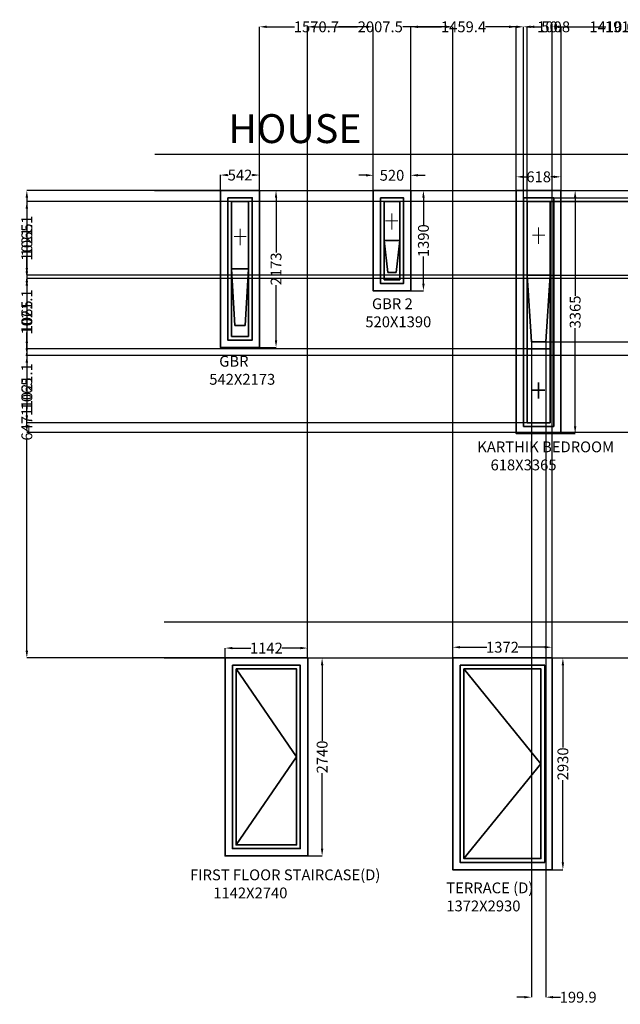
# Model space of a CAD drawing. Units: millimetres. Extents: x 16338 to 57165, y -4429 to 26237.
# Tile 1 of 6: x 16338 to 24645, y -4429 to 9199. Entities that reach past the tile are written whole.
import ezdxf

# ---------------------------------------------------------------- set-up
doc = ezdxf.new("R2010")
doc.units = ezdxf.units.MM
doc.header["$MEASUREMENT"] = 0
for name, color, linetype, lineweight in [('A-ANNO-DIMS', 5, 'Continuous', 18), ('A-ANNO-SYMB', 4, 'Continuous', 18), ('A-ANNO-TEXT', 3, 'Continuous', 18), ('A-ELEV', 8, 'Continuous', 25), ('A-GLAZ', 7, 'Continuous', 35)]:
    doc.layers.add(name, color=color, linetype=linetype, lineweight=lineweight)
doc.styles.get("Standard").update_dxf_attribs({"font": 'arial.ttf'})
doc.dimstyles.get("Standard").update_dxf_attribs({"dimtxt": 150, "dimasz": 100, "dimexe": 0.18, "dimexo": 0.0625, "dimgap": 0.09, "dimtad": 0, "dimdec": 0, "dimzin": 0, "dimdsep": 46, "dimtxsty": 'Standard', "dimcen": 0.09, "dimadec": 0, "dimazin": 0, "dimtfac": 1, "dimtdec": 0, "dimtofl": 0, "dimtmove": 0, "dimatfit": 3, "dimfxl": 1, "dimtolj": 1, "dimtzin": 0, "dimarcsym": 0})

# ---------------------------------------------------------------- blocks, each defined once
blk = doc.blocks.new('*D48')
at = {"layer": 'A-ANNO-DIMS', "color": 0, "lineweight": -2, "transparency": 16777216}
for p, q in [((19114, 6835), (19114, 7049)), ((19214, 7048), (19220, 7048)), ((19556, 7048), (19551, 7048)), ((19656, 6835), (19656, 7049))]:
    blk.add_line(p, q, dxfattribs=at)
at = {"layer": 'A-ANNO-DIMS', "color": 0, "transparency": 16777216}
for points in [[(19214, 7065), (19214, 7032), (19114, 7048)], [(19556, 7065), (19556, 7032), (19656, 7048)]]:
    blk.add_solid(points, dxfattribs=at)
at = {"layer": 'Defpoints', "color": 0, "transparency": 16777216}
for p in [(19656, 7048), (19114, 6835), (19656, 6835)]:
    blk.add_point(p, dxfattribs=at)
at = {"layer": 'A-ANNO-DIMS', "color": 0, "transparency": 16777216, "insert": (19385, 7048), "char_height": 150, "attachment_point": 5}
blk.add_mtext('\\A1;542', dxfattribs=at)
blk = doc.blocks.new('*D49')
at = {"layer": 'A-ANNO-DIMS', "color": 0, "lineweight": -2, "transparency": 16777216}
for p, q in [((19657, 6835), (19884, 6835)), ((19884, 6735), (19884, 5974)), ((19884, 4762), (19884, 5523)), ((19657, 4662), (19884, 4662))]:
    blk.add_line(p, q, dxfattribs=at)
at = {"layer": 'A-ANNO-DIMS', "color": 0, "transparency": 16777216}
for points in [[(19867, 6735), (19900, 6735), (19884, 6835)], [(19867, 4762), (19900, 4762), (19884, 4662)]]:
    blk.add_solid(points, dxfattribs=at)
at = {"layer": 'Defpoints', "color": 0, "transparency": 16777216}
for p in [(19656, 6835), (19656, 4662), (19884, 4662)]:
    blk.add_point(p, dxfattribs=at)
at = {"layer": 'A-ANNO-DIMS', "color": 0, "transparency": 16777216, "insert": (19884, 5749), "char_height": 150, "attachment_point": 5, "rotation": 90}
blk.add_mtext('\\A1;2173', dxfattribs=at)
blk = doc.blocks.new('*D50')
at = {"layer": 'A-ANNO-DIMS', "color": 0, "lineweight": -2, "transparency": 16777216}
for p, q in [((21127, 7045), (21027, 7045)), ((21227, 6835), (21227, 7045)), ((21747, 6835), (21747, 7045)), ((21847, 7045), (21947, 7045))]:
    blk.add_line(p, q, dxfattribs=at)
at = {"layer": 'A-ANNO-DIMS', "color": 0, "transparency": 16777216}
for points in [[(21127, 7062), (21127, 7028), (21227, 7045)], [(21847, 7062), (21847, 7028), (21747, 7045)]]:
    blk.add_solid(points, dxfattribs=at)
at = {"layer": 'Defpoints', "color": 0, "transparency": 16777216}
for p in [(21747, 7045), (21227, 6835), (21747, 6835)]:
    blk.add_point(p, dxfattribs=at)
at = {"layer": 'A-ANNO-DIMS', "color": 0, "transparency": 16777216, "insert": (21487, 7045), "char_height": 150, "attachment_point": 5}
blk.add_mtext('\\A1;520', dxfattribs=at)
blk = doc.blocks.new('*D51')
at = {"layer": 'A-ANNO-DIMS', "color": 0, "lineweight": -2, "transparency": 16777216}
for p, q in [((21747, 6835), (21923, 6835)), ((21922, 6735), (21922, 6357)), ((21922, 5545), (21922, 5923)), ((21747, 5445), (21923, 5445))]:
    blk.add_line(p, q, dxfattribs=at)
at = {"layer": 'A-ANNO-DIMS', "color": 0, "transparency": 16777216}
for points in [[(21906, 6735), (21939, 6735), (21922, 6835)], [(21906, 5545), (21939, 5545), (21922, 5445)]]:
    blk.add_solid(points, dxfattribs=at)
at = {"layer": 'Defpoints', "color": 0, "transparency": 16777216}
for p in [(21747, 6835), (21747, 5445), (21922, 5445)]:
    blk.add_point(p, dxfattribs=at)
at = {"layer": 'A-ANNO-DIMS', "color": 0, "transparency": 16777216, "insert": (21922, 6140), "char_height": 150, "attachment_point": 5, "rotation": 90}
blk.add_mtext('\\A1;1390', dxfattribs=at)
blk = doc.blocks.new('*D52')
at = {"layer": 'A-ANNO-DIMS', "color": 0, "lineweight": -2, "transparency": 16777216}
for p, q in [((23207, 6835), (23207, 7024)), ((23307, 7024), (23349, 7024)), ((23725, 7024), (23682, 7024)), ((23825, 6835), (23825, 7024))]:
    blk.add_line(p, q, dxfattribs=at)
at = {"layer": 'A-ANNO-DIMS', "color": 0, "transparency": 16777216}
for points in [[(23307, 7040), (23307, 7007), (23207, 7024)], [(23725, 7040), (23725, 7007), (23825, 7024)]]:
    blk.add_solid(points, dxfattribs=at)
at = {"layer": 'Defpoints', "color": 0, "transparency": 16777216}
for p in [(23825, 7024), (23207, 6835), (23825, 6835)]:
    blk.add_point(p, dxfattribs=at)
at = {"layer": 'A-ANNO-DIMS', "color": 0, "transparency": 16777216, "insert": (23516, 7024), "char_height": 150, "attachment_point": 5}
blk.add_mtext('\\A1;618', dxfattribs=at)
blk = doc.blocks.new('*D53')
at = {"layer": 'A-ANNO-DIMS', "color": 0, "lineweight": -2, "transparency": 16777216}
for p, q in [((23825, 6835), (24021, 6835)), ((24021, 6735), (24021, 5377)), ((24021, 3570), (24021, 4928)), ((23825, 3470), (24021, 3470))]:
    blk.add_line(p, q, dxfattribs=at)
at = {"layer": 'A-ANNO-DIMS', "color": 0, "transparency": 16777216}
for points in [[(24004, 6735), (24037, 6735), (24021, 6835)], [(24004, 3570), (24037, 3570), (24021, 3470)]]:
    blk.add_solid(points, dxfattribs=at)
at = {"layer": 'Defpoints', "color": 0, "transparency": 16777216}
for p in [(23825, 6835), (23825, 3470), (24021, 3470)]:
    blk.add_point(p, dxfattribs=at)
at = {"layer": 'A-ANNO-DIMS', "color": 0, "transparency": 16777216, "insert": (24021, 5153), "char_height": 150, "attachment_point": 5, "rotation": 90}
blk.add_mtext('\\A1;3365', dxfattribs=at)
blk = doc.blocks.new('*D71')
at = {"layer": 'A-ANNO-DIMS', "color": 0, "lineweight": -2, "transparency": 16777216}
for p, q in [((19179, 364), (19179, 501)), ((19279, 501), (19534, 501)), ((20221, 501), (19966, 501)), ((20321, 364), (20321, 501))]:
    blk.add_line(p, q, dxfattribs=at)
at = {"layer": 'A-ANNO-DIMS', "color": 0, "transparency": 16777216}
for points in [[(19279, 518), (19279, 485), (19179, 501)], [(20221, 518), (20221, 485), (20321, 501)]]:
    blk.add_solid(points, dxfattribs=at)
at = {"layer": 'Defpoints', "color": 0, "transparency": 16777216}
for p in [(20321, 501), (19179, 364), (20321, 364)]:
    blk.add_point(p, dxfattribs=at)
at = {"layer": 'A-ANNO-DIMS', "color": 0, "transparency": 16777216, "insert": (19750, 501), "char_height": 150, "attachment_point": 5}
blk.add_mtext('\\A1;1142', dxfattribs=at)
blk = doc.blocks.new('*D72')
at = {"layer": 'A-ANNO-DIMS', "color": 0, "lineweight": -2, "transparency": 16777216}
for p, q in [((20321, 364), (20521, 364)), ((20521, 264), (20521, -781)), ((20521, -2276), (20521, -1231)), ((20321, -2376), (20521, -2376))]:
    blk.add_line(p, q, dxfattribs=at)
at = {"layer": 'A-ANNO-DIMS', "color": 0, "transparency": 16777216}
for points in [[(20504, 264), (20538, 264), (20521, 364)], [(20504, -2276), (20538, -2276), (20521, -2376)]]:
    blk.add_solid(points, dxfattribs=at)
at = {"layer": 'Defpoints', "color": 0, "transparency": 16777216}
for p in [(20321, 364), (20321, -2376), (20521, -2376)]:
    blk.add_point(p, dxfattribs=at)
at = {"layer": 'A-ANNO-DIMS', "color": 0, "transparency": 16777216, "insert": (20521, -1006), "char_height": 150, "attachment_point": 5, "rotation": 90}
blk.add_mtext('\\A1;2740', dxfattribs=at)
blk = doc.blocks.new('*D73')
at = {"layer": 'A-ANNO-DIMS', "color": 0, "lineweight": -2, "transparency": 16777216}
for p, q in [((22329, 364), (22329, 513)), ((22429, 513), (22798, 513)), ((23601, 513), (23231, 513)), ((23701, 364), (23701, 513))]:
    blk.add_line(p, q, dxfattribs=at)
at = {"layer": 'A-ANNO-DIMS', "color": 0, "transparency": 16777216}
for points in [[(22429, 529), (22429, 496), (22329, 513)], [(23601, 529), (23601, 496), (23701, 513)]]:
    blk.add_solid(points, dxfattribs=at)
at = {"layer": 'Defpoints', "color": 0, "transparency": 16777216}
for p in [(23701, 513), (22329, 364), (23701, 364)]:
    blk.add_point(p, dxfattribs=at)
at = {"layer": 'A-ANNO-DIMS', "color": 0, "transparency": 16777216, "insert": (23015, 513), "char_height": 150, "attachment_point": 5}
blk.add_mtext('\\A1;1372', dxfattribs=at)
blk = doc.blocks.new('*D74')
at = {"layer": 'A-ANNO-DIMS', "color": 0, "lineweight": -2, "transparency": 16777216}
for p, q in [((23701, 364), (23851, 364)), ((23851, 264), (23851, -876)), ((23851, -2466), (23851, -1326)), ((23701, -2566), (23851, -2566))]:
    blk.add_line(p, q, dxfattribs=at)
at = {"layer": 'A-ANNO-DIMS', "color": 0, "transparency": 16777216}
for points in [[(23834, 264), (23867, 264), (23851, 364)], [(23834, -2466), (23867, -2466), (23851, -2566)]]:
    blk.add_solid(points, dxfattribs=at)
at = {"layer": 'Defpoints', "color": 0, "transparency": 16777216}
for p in [(23701, 364), (23701, -2566), (23851, -2566)]:
    blk.add_point(p, dxfattribs=at)
at = {"layer": 'A-ANNO-DIMS', "color": 0, "transparency": 16777216, "insert": (23851, -1101), "char_height": 150, "attachment_point": 5, "rotation": 90}
blk.add_mtext('\\A1;2930', dxfattribs=at)
blk = doc.blocks.new('*D107')
at = {"layer": 'A-ANNO-DIMS', "color": 0, "lineweight": -2, "transparency": 16777216}
for p, q in [((19656, 6835), (19656, 9100)), ((19756, 9100), (20137, 9100)), ((21127, 9100), (20746, 9100)), ((21227, 6835), (21227, 9100))]:
    blk.add_line(p, q, dxfattribs=at)
at = {"layer": 'A-ANNO-DIMS', "color": 0, "transparency": 16777216}
for points in [[(19756, 9117), (19756, 9083), (19656, 9100)], [(21127, 9117), (21127, 9083), (21227, 9100)]]:
    blk.add_solid(points, dxfattribs=at)
at = {"layer": 'Defpoints', "color": 0, "transparency": 16777216}
for p in [(21227, 9100), (19656, 6835), (21227, 6835)]:
    blk.add_point(p, dxfattribs=at)
at = {"layer": 'A-ANNO-DIMS', "color": 0, "transparency": 16777216, "insert": (20442, 9100), "char_height": 150, "attachment_point": 5}
blk.add_mtext('\\A1;1570.7', dxfattribs=at)
blk = doc.blocks.new('*D108')
at = {"layer": 'A-ANNO-DIMS', "color": 0, "lineweight": -2, "transparency": 16777216}
for p, q in [((21747, 6835), (21747, 9100)), ((21847, 9100), (22173, 9100)), ((23107, 9100), (22781, 9100)), ((23207, 6835), (23207, 9100))]:
    blk.add_line(p, q, dxfattribs=at)
at = {"layer": 'A-ANNO-DIMS', "color": 0, "transparency": 16777216}
for points in [[(21847, 9117), (21847, 9083), (21747, 9100)], [(23107, 9117), (23107, 9083), (23207, 9100)]]:
    blk.add_solid(points, dxfattribs=at)
at = {"layer": 'Defpoints', "color": 0, "transparency": 16777216}
for p in [(23207, 9100), (21747, 6835), (23207, 6835)]:
    blk.add_point(p, dxfattribs=at)
at = {"layer": 'A-ANNO-DIMS', "color": 0, "transparency": 16777216, "insert": (22477, 9100), "char_height": 150, "attachment_point": 5}
blk.add_mtext('\\A1;1459.4', dxfattribs=at)
blk = doc.blocks.new('*D109')
at = {"layer": 'A-ANNO-DIMS', "color": 0, "lineweight": -2, "transparency": 16777216}
for p, q in [((23825, 6835), (23825, 9100)), ((23925, 9100), (24226, 9100)), ((25135, 9100), (24834, 9100)), ((25235, 6835), (25235, 9100))]:
    blk.add_line(p, q, dxfattribs=at)
at = {"layer": 'A-ANNO-DIMS', "color": 0, "transparency": 16777216}
for points in [[(23925, 9117), (23925, 9083), (23825, 9100)], [(25135, 9117), (25135, 9083), (25235, 9100)]]:
    blk.add_solid(points, dxfattribs=at)
at = {"layer": 'Defpoints', "color": 0, "transparency": 16777216}
for p in [(25235, 9100), (23825, 6835), (25235, 6835)]:
    blk.add_point(p, dxfattribs=at)
at = {"layer": 'A-ANNO-DIMS', "color": 0, "transparency": 16777216, "insert": (24530, 9100), "char_height": 150, "attachment_point": 5}
blk.add_mtext('\\A1;1410.6', dxfattribs=at)
blk = doc.blocks.new('*D118')
at = {"layer": 'A-ANNO-DIMS', "color": 0, "lineweight": -2, "transparency": 16777216}
for p, q in [((20321, 364), (20321, 9100)), ((20421, 9100), (21012, 9100)), ((22229, 9100), (21638, 9100)), ((22329, 364), (22329, 9100))]:
    blk.add_line(p, q, dxfattribs=at)
at = {"layer": 'A-ANNO-DIMS', "color": 0, "transparency": 16777216}
for points in [[(20421, 9117), (20421, 9083), (20321, 9100)], [(22229, 9117), (22229, 9083), (22329, 9100)]]:
    blk.add_solid(points, dxfattribs=at)
at = {"layer": 'Defpoints', "color": 0, "transparency": 16777216}
for p in [(22329, 9100), (20321, 364), (22329, 364)]:
    blk.add_point(p, dxfattribs=at)
at = {"layer": 'A-ANNO-DIMS', "color": 0, "transparency": 16777216, "insert": (21325, 9100), "char_height": 150, "attachment_point": 5}
blk.add_mtext('\\A1;2007.5', dxfattribs=at)
blk = doc.blocks.new('*D119')
at = {"layer": 'A-ANNO-DIMS', "color": 0, "lineweight": -2, "transparency": 16777216}
for p, q in [((23701, 364), (23701, 9100)), ((23801, 9100), (24443, 9100)), ((25520, 9100), (24877, 9100)), ((25620, 364), (25620, 9100))]:
    blk.add_line(p, q, dxfattribs=at)
at = {"layer": 'A-ANNO-DIMS', "color": 0, "transparency": 16777216}
for points in [[(23801, 9117), (23801, 9083), (23701, 9100)], [(25520, 9117), (25520, 9083), (25620, 9100)]]:
    blk.add_solid(points, dxfattribs=at)
at = {"layer": 'Defpoints', "color": 0, "transparency": 16777216}
for p in [(25620, 9100), (23701, 364), (25620, 364)]:
    blk.add_point(p, dxfattribs=at)
at = {"layer": 'A-ANNO-DIMS', "color": 0, "transparency": 16777216, "insert": (24660, 9100), "char_height": 150, "attachment_point": 5}
blk.add_mtext('\\A1;1919', dxfattribs=at)
blk = doc.blocks.new('*D120')
at = {"layer": 'A-ANNO-DIMS', "color": 0, "lineweight": -2, "transparency": 16777216}
for p, q in [((19114, 6835), (16437, 6835)), ((16437, 6735), (16437, 3810)), ((16437, 464), (16437, 3390)), ((19179, 364), (16437, 364))]:
    blk.add_line(p, q, dxfattribs=at)
at = {"layer": 'A-ANNO-DIMS', "color": 0, "transparency": 16777216}
for points in [[(16420, 6735), (16454, 6735), (16437, 6835)], [(16420, 464), (16454, 464), (16437, 364)]]:
    blk.add_solid(points, dxfattribs=at)
at = {"layer": 'Defpoints', "color": 0, "transparency": 16777216}
for p in [(19114, 6835), (16437, 364), (19179, 364)]:
    blk.add_point(p, dxfattribs=at)
at = {"layer": 'A-ANNO-DIMS', "color": 0, "transparency": 16777216, "insert": (16437, 3600), "char_height": 150, "attachment_point": 5, "rotation": 90}
blk.add_mtext('\\A1;6471', dxfattribs=at)
blk = doc.blocks.new('*D121')
at = {"layer": 'A-ANNO-DIMS', "color": 0, "lineweight": -2, "transparency": 16777216}
for p, q in [((27066, 6682), (16437, 6682)), ((16437, 6582), (16437, 6367)), ((16437, 5717), (16437, 5932)), ((27066, 5617), (16437, 5617))]:
    blk.add_line(p, q, dxfattribs=at)
at = {"layer": 'A-ANNO-DIMS', "color": 0, "transparency": 16777216}
for points in [[(16420, 6582), (16454, 6582), (16437, 6682)], [(16420, 5717), (16454, 5717), (16437, 5617)]]:
    blk.add_solid(points, dxfattribs=at)
at = {"layer": 'Defpoints', "color": 0, "transparency": 16777216}
for p in [(27066, 6682), (16437, 5617), (27066, 5617)]:
    blk.add_point(p, dxfattribs=at)
at = {"layer": 'A-ANNO-DIMS', "color": 0, "transparency": 16777216, "insert": (16437, 6150), "char_height": 150, "attachment_point": 5, "rotation": 90}
blk.add_mtext('\\A1;1065', dxfattribs=at)
blk = doc.blocks.new('*D122')
at = {"layer": 'A-ANNO-DIMS', "color": 0, "lineweight": -2, "transparency": 16777216}
for p, q in [((27066, 5617), (16437, 5617)), ((16437, 5517), (16437, 5302)), ((16437, 4652), (16437, 4867)), ((27066, 4552), (16437, 4552))]:
    blk.add_line(p, q, dxfattribs=at)
at = {"layer": 'A-ANNO-DIMS', "color": 0, "transparency": 16777216}
for points in [[(16420, 5517), (16454, 5517), (16437, 5617)], [(16420, 4652), (16454, 4652), (16437, 4552)]]:
    blk.add_solid(points, dxfattribs=at)
at = {"layer": 'Defpoints', "color": 0, "transparency": 16777216}
for p in [(27066, 5617), (16437, 4552), (27066, 4552)]:
    blk.add_point(p, dxfattribs=at)
at = {"layer": 'A-ANNO-DIMS', "color": 0, "transparency": 16777216, "insert": (16437, 5084), "char_height": 150, "attachment_point": 5, "rotation": 90}
blk.add_mtext('\\A1;1065', dxfattribs=at)
blk = doc.blocks.new('*D123')
at = {"layer": 'A-ANNO-DIMS', "color": 0, "lineweight": -2, "transparency": 16777216}
for p, q in [((27066, 4552), (16437, 4552)), ((16437, 4452), (16437, 4237)), ((16437, 3587), (16437, 3802)), ((27066, 3487), (16437, 3487))]:
    blk.add_line(p, q, dxfattribs=at)
at = {"layer": 'A-ANNO-DIMS', "color": 0, "transparency": 16777216}
for points in [[(16420, 4452), (16454, 4452), (16437, 4552)], [(16420, 3587), (16454, 3587), (16437, 3487)]]:
    blk.add_solid(points, dxfattribs=at)
at = {"layer": 'Defpoints', "color": 0, "transparency": 16777216}
for p in [(27066, 4552), (16437, 3487), (27066, 3487)]:
    blk.add_point(p, dxfattribs=at)
at = {"layer": 'A-ANNO-DIMS', "color": 0, "transparency": 16777216, "insert": (16437, 4019), "char_height": 150, "attachment_point": 5, "rotation": 90}
blk.add_mtext('\\A1;1065', dxfattribs=at)
blk = doc.blocks.new('*D124')
at = {"layer": 'A-ANNO-DIMS', "color": 0, "lineweight": -2, "transparency": 16777216}
for p, q in [((23107, 9100), (23007, 9100)), ((23207, 6835), (23207, 9100)), ((23307, 6735), (23307, 9100)), ((23407, 9100), (23507, 9100))]:
    blk.add_line(p, q, dxfattribs=at)
at = {"layer": 'A-ANNO-DIMS', "color": 0, "transparency": 16777216}
for points in [[(23107, 9117), (23107, 9083), (23207, 9100)], [(23407, 9117), (23407, 9083), (23307, 9100)]]:
    blk.add_solid(points, dxfattribs=at)
at = {"layer": 'Defpoints', "color": 0, "transparency": 16777216}
for p in [(23307, 9100), (23207, 6835), (23307, 6735)]:
    blk.add_point(p, dxfattribs=at)
at = {"layer": 'A-ANNO-DIMS', "color": 0, "transparency": 16777216, "insert": (23665, 9100), "char_height": 150, "attachment_point": 5}
blk.add_mtext('\\A1;100', dxfattribs=at)
blk = doc.blocks.new('*D125')
at = {"layer": 'A-ANNO-DIMS', "color": 0, "lineweight": -2, "transparency": 16777216}
for p, q in [((23207, 9100), (23107, 9100)), ((23307, 6735), (23307, 9100)), ((23357, 6684), (23357, 9100)), ((23457, 9100), (23557, 9100))]:
    blk.add_line(p, q, dxfattribs=at)
at = {"layer": 'A-ANNO-DIMS', "color": 0, "transparency": 16777216}
for points in [[(23207, 9117), (23207, 9083), (23307, 9100)], [(23457, 9117), (23457, 9083), (23357, 9100)]]:
    blk.add_solid(points, dxfattribs=at)
at = {"layer": 'Defpoints', "color": 0, "transparency": 16777216}
for p in [(23357, 9100), (23307, 6735), (23357, 6684)]:
    blk.add_point(p, dxfattribs=at)
at = {"layer": 'A-ANNO-DIMS', "color": 0, "transparency": 16777216, "insert": (23752, 9100), "char_height": 150, "attachment_point": 5}
blk.add_mtext('\\A1;50.8', dxfattribs=at)
blk = doc.blocks.new('*D126')
at = {"layer": 'A-ANNO-DIMS', "color": 0, "lineweight": -2, "transparency": 16777216}
for p, q in [((52648, 6935), (52648, 7035)), ((23825, 6835), (52648, 6835)), ((23725, 6735), (52648, 6735)), ((52648, 6635), (52648, 6535))]:
    blk.add_line(p, q, dxfattribs=at)
at = {"layer": 'A-ANNO-DIMS', "color": 0, "transparency": 16777216}
for points in [[(52631, 6935), (52665, 6935), (52648, 6835)], [(52631, 6635), (52665, 6635), (52648, 6735)]]:
    blk.add_solid(points, dxfattribs=at)
at = {"layer": 'Defpoints', "color": 0, "transparency": 16777216}
for p in [(23825, 6835), (23725, 6735), (52648, 6735)]:
    blk.add_point(p, dxfattribs=at)
at = {"layer": 'A-ANNO-DIMS', "color": 0, "transparency": 16777216, "insert": (52648, 6377), "char_height": 150, "attachment_point": 5, "rotation": 90}
blk.add_mtext('\\A1;100', dxfattribs=at)
blk = doc.blocks.new('*D127')
at = {"layer": 'A-ANNO-DIMS', "color": 0, "lineweight": -2, "transparency": 16777216}
for p, q in [((52648, 6835), (52648, 6935)), ((23674, 6684), (52648, 6684)), ((23725, 6735), (52648, 6735)), ((52648, 6584), (52648, 6484))]:
    blk.add_line(p, q, dxfattribs=at)
at = {"layer": 'A-ANNO-DIMS', "color": 0, "transparency": 16777216}
for points in [[(52631, 6835), (52665, 6835), (52648, 6735)], [(52631, 6584), (52665, 6584), (52648, 6684)]]:
    blk.add_solid(points, dxfattribs=at)
at = {"layer": 'Defpoints', "color": 0, "transparency": 16777216}
for p in [(23674, 6684), (23725, 6735), (52648, 6684)]:
    blk.add_point(p, dxfattribs=at)
at = {"layer": 'A-ANNO-DIMS', "color": 0, "transparency": 16777216, "insert": (52648, 6289), "char_height": 150, "attachment_point": 5, "rotation": 90}
blk.add_mtext('\\A1;50.8', dxfattribs=at)
blk = doc.blocks.new('*D128')
at = {"layer": 'A-ANNO-DIMS', "color": 0, "lineweight": -2, "transparency": 16777216}
for p, q in [((23357, 6684), (16437, 6684)), ((16437, 6584), (16437, 6464)), ((16437, 5763), (16437, 5884)), ((23357, 5663), (16437, 5663))]:
    blk.add_line(p, q, dxfattribs=at)
at = {"layer": 'A-ANNO-DIMS', "color": 0, "transparency": 16777216}
for points in [[(16420, 6584), (16454, 6584), (16437, 6684)], [(16420, 5763), (16454, 5763), (16437, 5663)]]:
    blk.add_solid(points, dxfattribs=at)
at = {"layer": 'Defpoints', "color": 0, "transparency": 16777216}
for p in [(23357, 6684), (16437, 5663), (23357, 5663)]:
    blk.add_point(p, dxfattribs=at)
at = {"layer": 'A-ANNO-DIMS', "color": 0, "transparency": 16777216, "insert": (16437, 6174), "char_height": 150, "attachment_point": 5, "rotation": 90}
blk.add_mtext('\\A1;1021.1', dxfattribs=at)
blk = doc.blocks.new('*D129')
at = {"layer": 'A-ANNO-DIMS', "color": 0, "lineweight": -2, "transparency": 16777216}
for p, q in [((23357, 5663), (16437, 5663)), ((16437, 5563), (16437, 5443)), ((16437, 4742), (16437, 4863)), ((23357, 4642), (16437, 4642))]:
    blk.add_line(p, q, dxfattribs=at)
at = {"layer": 'A-ANNO-DIMS', "color": 0, "transparency": 16777216}
for points in [[(16420, 5563), (16454, 5563), (16437, 5663)], [(16420, 4742), (16454, 4742), (16437, 4642)]]:
    blk.add_solid(points, dxfattribs=at)
at = {"layer": 'Defpoints', "color": 0, "transparency": 16777216}
for p in [(23357, 5663), (16437, 4642), (23357, 4642)]:
    blk.add_point(p, dxfattribs=at)
at = {"layer": 'A-ANNO-DIMS', "color": 0, "transparency": 16777216, "insert": (16437, 5153), "char_height": 150, "attachment_point": 5, "rotation": 90}
blk.add_mtext('\\A1;1021.1', dxfattribs=at)
blk = doc.blocks.new('*D130')
at = {"layer": 'A-ANNO-DIMS', "color": 0, "lineweight": -2, "transparency": 16777216}
for p, q in [((23357, 4642), (16437, 4642)), ((16437, 4542), (16437, 4421)), ((16437, 3721), (16437, 3842)), ((23357, 3621), (16437, 3621))]:
    blk.add_line(p, q, dxfattribs=at)
at = {"layer": 'A-ANNO-DIMS', "color": 0, "transparency": 16777216}
for points in [[(16420, 4542), (16454, 4542), (16437, 4642)], [(16420, 3721), (16454, 3721), (16437, 3621)]]:
    blk.add_solid(points, dxfattribs=at)
at = {"layer": 'Defpoints', "color": 0, "transparency": 16777216}
for p in [(23357, 4642), (16437, 3621), (23357, 3621)]:
    blk.add_point(p, dxfattribs=at)
at = {"layer": 'A-ANNO-DIMS', "color": 0, "transparency": 16777216, "insert": (16437, 4131), "char_height": 150, "attachment_point": 5, "rotation": 90}
blk.add_mtext('\\A1;1021.1', dxfattribs=at)
blk = doc.blocks.new('*D131')
at = {"layer": 'A-ANNO-DIMS', "color": 0, "lineweight": -2, "transparency": 16777216}
for p, q in [((23416, 4742), (23416, -4331)), ((23616, 4742), (23616, -4331)), ((23316, -4331), (23216, -4331)), ((23716, -4331), (23816, -4331))]:
    blk.add_line(p, q, dxfattribs=at)
at = {"layer": 'A-ANNO-DIMS', "color": 0, "transparency": 16777216}
for points in [[(23316, -4314), (23316, -4348), (23416, -4331)], [(23716, -4314), (23716, -4348), (23616, -4331)]]:
    blk.add_solid(points, dxfattribs=at)
at = {"layer": 'Defpoints', "color": 0, "transparency": 16777216}
for p in [(23416, 4742), (23616, 4742), (23616, -4331)]:
    blk.add_point(p, dxfattribs=at)
at = {"layer": 'A-ANNO-DIMS', "color": 0, "transparency": 16777216, "insert": (24062, -4331), "char_height": 150, "attachment_point": 5}
blk.add_mtext('\\A1;199.9', dxfattribs=at)
blk = doc.blocks.new('*D132')
at = {"layer": 'A-ANNO-DIMS', "color": 0, "lineweight": -2, "transparency": 16777216}
for p, q in [((23674, 5663), (52648, 5663)), ((52648, 5563), (52648, 5441)), ((52648, 4842), (52648, 4964)), ((23616, 4742), (52648, 4742))]:
    blk.add_line(p, q, dxfattribs=at)
at = {"layer": 'A-ANNO-DIMS', "color": 0, "transparency": 16777216}
for points in [[(52631, 5563), (52665, 5563), (52648, 5663)], [(52631, 4842), (52665, 4842), (52648, 4742)]]:
    blk.add_solid(points, dxfattribs=at)
at = {"layer": 'Defpoints', "color": 0, "transparency": 16777216}
for p in [(23674, 5663), (52648, 5663), (23616, 4742)]:
    blk.add_point(p, dxfattribs=at)
at = {"layer": 'A-ANNO-DIMS', "color": 0, "transparency": 16777216, "insert": (52648, 5203), "char_height": 150, "attachment_point": 5, "rotation": 90}
blk.add_mtext('\\A1;921.1', dxfattribs=at)

msp = doc.modelspace()

# ---------------------------------------------------------------- linework, layer by layer
at = {"layer": 'A-ANNO-DIMS'}
for p in [(23357.39, 5663.17), (23357.39, 4642.04)]:
    msp.add_point(p, dxfattribs=at)
at = {"layer": 'A-ANNO-SYMB'}
for p, q in [((21399.7, 6412.56), (21569.55, 6412.56)), ((21484.62, 6293.3), (21484.62, 6515.75)), ((19387.32, 6079.71), (19387.32, 6302.16)), ((23514.15, 6098.5), (23514.15, 6320.95)), ((19302.4, 6198.96), (19472.25, 6198.96)), ((23429.22, 6217.75), (23599.07, 6217.75))]:
    msp.add_line(p, q, dxfattribs=at)
at = {"layer": 'A-ELEV'}
for p, q in [((18209.23, 7335.1), (50757.08, 7335.1)), ((18201.83, 6834.85), (50882.91, 6829.39)), ((18334.8, 864.14), (29883.27, 864.14)), ((18334.8, 364.14), (29883.27, 364.14))]:
    msp.add_line(p, q, dxfattribs=at)
at = {"layer": 'A-GLAZ'}
for p, q in [((19266.88, 6682.7), (19504.08, 6682.7)), ((19266.88, 4814.5), (19266.88, 6682.7)), ((19504.08, 6682.7), (19504.08, 4814.5)), ((21379.55, 6682.7), (21594.75, 6682.7)), ((21379.55, 5597.5), (21379.55, 6682.7)), ((21594.75, 6682.7), (21594.75, 5597.5)), ((23357.39, 6684.3), (23673.79, 6684.3)), ((23357.39, 3620.9), (23357.39, 6684.3)), ((23673.79, 6684.3), (23673.79, 3620.9)), ((21379.55, 6140.1), (21594.75, 6140.1)), ((21379.55, 6140.1), (21428.46, 5697.5)), ((21594.75, 6140.1), (21545.84, 5697.5)), ((19266.88, 5748.6), (19504.08, 5748.6)), ((19266.88, 5748.6), (19314.53, 4964.5)), ((19504.08, 5748.6), (19456.43, 4964.5)), ((21594.75, 5597.5), (21379.55, 5597.5)), ((21545.84, 5697.5), (21428.46, 5697.5)), ((23357.39, 5663.17), (23673.79, 5663.17)), ((23357.39, 5663.17), (23415.63, 4742.04)), ((23673.79, 5663.17), (23615.55, 4742.04)), ((19456.43, 4964.5), (19314.53, 4964.5)), ((19504.08, 4814.5), (19266.88, 4814.5)), ((23357.39, 4642.04), (23673.79, 4642.04)), ((23415.63, 4742.04), (23615.55, 4742.04)), ((23514.15, 3953.92), (23514.15, 4176.37)), ((23429.22, 4073.18), (23599.07, 4073.18)), ((23673.79, 3620.9), (23357.39, 3620.9)), ((19331.57, 211.74), (20168.77, -1005.86)), ((22481.07, 211.74), (23548.27, -1100.86)), ((20168.77, -1005.86), (19331.57, -2223.46)), ((23548.27, -1100.86), (22481.07, -2413.46))]:
    msp.add_line(p, q, dxfattribs=at)
for points in [[(19114.48, 6835.1), (19656.48, 6835.1), (19656.48, 4662.1), (19114.48, 4662.1)], [(21227.15, 6835.1), (21747.15, 6835.1), (21747.15, 5445.1), (21227.15, 5445.1)], [(23206.59, 6835.1), (23824.59, 6835.1), (23824.59, 3470.1), (23206.59, 3470.1)], [(19216.08, 6733.5), (19554.88, 6733.5), (19554.88, 4763.7), (19216.08, 4763.7)], [(21328.75, 6733.5), (21645.55, 6733.5), (21645.55, 5546.7), (21328.75, 5546.7)], [(23306.59, 6735.1), (23724.59, 6735.1), (23724.59, 3570.1), (23306.59, 3570.1)], [(19179.17, 364.14), (20321.17, 364.14), (20321.17, -2375.86), (19179.17, -2375.86)], [(22328.67, 364.14), (23700.67, 364.14), (23700.67, -2565.86), (22328.67, -2565.86)], [(19280.77, 262.54), (20219.57, 262.54), (20219.57, -2274.26), (19280.77, -2274.26)], [(19331.57, 211.74), (20168.77, 211.74), (20168.77, -2223.46), (19331.57, -2223.46)], [(22430.27, 262.54), (23599.07, 262.54), (23599.07, -2464.26), (22430.27, -2464.26)], [(22481.07, 211.74), (23548.27, 211.74), (23548.27, -2413.46), (22481.07, -2413.46)]]:
    msp.add_lwpolyline(points, close=True, dxfattribs=at)

# ---------------------------------------------------------------- texts
at = {"layer": 'A-ANNO-TEXT', "attachment_point": 1}
for s, insert, char_height in [('HOUSE', (19224.15, 7890.8), 400), ('  GBR 2\\P520X1390', (21118.55, 5341.73), 150), ('   GBR\\P542X2173', (18959.98, 4546.18), 150), ('KARTHIK BEDROOM\\P    618X3365', (22667.22, 3361.15), 150), ('FIRST FLOOR STAIRCASE(D)\\P       1142X2740', (18694.45, -2562.66), 150), ('TERRACE (D)\\P1372X2930', (22238.72, -2742.83), 150)]:
    msp.add_mtext_dynamic_manual_height_columns(s, width=7094.9176, gutter_width=1, heights=[0], dxfattribs=dict(at, insert=insert, char_height=char_height))

# ---------------------------------------------------------------- dimensions: what is measured, and where the dimension line sits
at = {"layer": 'A-ANNO-DIMS'}
for base, p1, p2, override, picture, middle in [((21227.15, 9100.1), (19656.48, 6835.1), (21227.15, 6835.1), {"dimdec": 1, "dimlfac": 1, "dimrnd": 0, "dimzin": 0, "dimdsep": 46, "dimlunit": 2}, '*D107', (20441.81, 9100.1)), ((22328.67, 9100.1), (20321.17, 364.14), (22328.67, 364.14), {"dimdec": 1, "dimlfac": 1, "dimrnd": 0, "dimzin": 0, "dimdsep": 46, "dimlunit": 2}, '*D118', (21324.92, 9100.1)), ((23206.59, 9100.1), (21747.15, 6835.1), (23206.59, 6835.1), {"dimdec": 1, "dimlfac": 1, "dimrnd": 0, "dimzin": 0, "dimdsep": 46, "dimlunit": 2}, '*D108', (22476.87, 9100.1)), ((23306.59, 9100.1), (23206.59, 6835.1), (23306.59, 6735.1), {"dimdec": 0, "dimlfac": 1, "dimrnd": 0, "dimzin": 0, "dimdsep": 46, "dimlunit": 2}, '*D124', (23665.07, 9100.1)), ((23357.39, 9100.1), (23306.59, 6735.1), (23357.39, 6684.3), {"dimdec": 1, "dimlfac": 1, "dimrnd": 0, "dimzin": 0, "dimdsep": 46, "dimlunit": 2}, '*D125', (23752.45, 9100.1)), ((25619.75, 9100.1), (23700.67, 364.14), (25619.75, 364.14), {"dimdec": 0, "dimlfac": 1, "dimrnd": 0, "dimzin": 0, "dimdsep": 46, "dimlunit": 2}, '*D119', (24660.21, 9100.1)), ((25235.23, 9100.1), (23824.59, 6835.1), (25235.23, 6835.1), {"dimdec": 1, "dimlfac": 1, "dimrnd": 0, "dimzin": 0, "dimdsep": 46, "dimlunit": 2}, '*D109', (24529.91, 9100.1)), ((19656.48, 7048.4), (19114.48, 6835.1), (19656.48, 6835.1), {"dimclrd": 0, "dimclre": 0, "dimclrt": 0}, '*D48', (19385.48, 7048.4)), ((21747.15, 7045.14), (21227.15, 6835.1), (21747.15, 6835.1), {"dimclrd": 0, "dimclre": 0, "dimclrt": 0}, '*D50', (21487.15, 7045.14)), ((23824.59, 7023.56), (23206.59, 6835.1), (23824.59, 6835.1), {"dimclrd": 0, "dimclre": 0, "dimclrt": 0}, '*D52', (23515.59, 7023.56)), ((23615.55, -4330.86), (23415.63, 4742.04), (23615.55, 4742.04), {"dimdec": 1, "dimlfac": 1, "dimrnd": 0, "dimzin": 0, "dimdsep": 46, "dimlunit": 2}, '*D131', (24061.82, -4330.86)), ((20321.17, 501.28), (19179.17, 364.14), (20321.17, 364.14), {"dimclrd": 0, "dimclre": 0, "dimclrt": 0}, '*D71', (19750.17, 501.28)), ((23700.67, 512.6), (22328.67, 364.14), (23700.67, 364.14), {"dimclrd": 0, "dimclre": 0, "dimclrt": 0}, '*D73', (23014.67, 512.6))]:
    dim = msp.add_linear_dim(base=base, p1=p1, p2=p2, dimstyle='Standard', override=override, dxfattribs=at)
    dim.commit()
    dim.dimension.update_dxf_attribs({"geometry": picture, "text_midpoint": middle})
for base, p1, p2, override, picture, middle in [((52647.91, 6735.1), (23824.59, 6835.1), (23724.59, 6735.1), {"dimdec": 0, "dimlfac": 1, "dimrnd": 0, "dimzin": 0, "dimdsep": 46, "dimlunit": 2}, '*D126', (52647.91, 6376.62)), ((16436.83, 364.14), (19114.48, 6835.1), (19179.17, 364.14), {"dimdec": 0, "dimlfac": 1, "dimrnd": 0, "dimzin": 0, "dimdsep": 46, "dimlunit": 2}, '*D120', (16436.83, 3599.62)), ((19883.58, 4662.1), (19656.48, 6835.1), (19656.48, 4662.1), {"dimclrd": 0, "dimclre": 0, "dimclrt": 0}, '*D49', (19883.58, 5748.6)), ((21922.32, 5445.1), (21747.15, 6835.1), (21747.15, 5445.1), {"dimclrd": 0, "dimclre": 0, "dimclrt": 0}, '*D51', (21922.32, 6140.1)), ((52647.91, 6684.3), (23724.59, 6735.1), (23673.79, 6684.3), {"dimdec": 1, "dimlfac": 1, "dimrnd": 0, "dimzin": 0, "dimdsep": 46, "dimlunit": 2}, '*D127', (52647.91, 6289.25)), ((24020.66, 3470.1), (23824.59, 6835.1), (23824.59, 3470.1), {"dimclrd": 0, "dimclre": 0, "dimclrt": 0}, '*D53', (24020.66, 5152.6)), ((16436.83, 5663.17), (23357.39, 6684.3), (23357.39, 5663.17), {"dimdec": 1, "dimlfac": 1, "dimrnd": 0, "dimzin": 0, "dimdsep": 46, "dimlunit": 2}, '*D128', (16436.83, 6173.74)), ((16436.83, 5617), (27065.98, 6682.06), (27065.98, 5617), {"dimdec": 0, "dimlfac": 1, "dimrnd": 0, "dimzin": 0, "dimdsep": 46, "dimlunit": 2}, '*D121', (16436.83, 6149.53)), ((16436.83, 4642.04), (23357.39, 5663.17), (23357.39, 4642.04), {"dimdec": 1, "dimlfac": 1, "dimrnd": 0, "dimzin": 0, "dimdsep": 46, "dimlunit": 2}, '*D129', (16436.83, 5152.6)), ((16436.83, 4551.93), (27065.98, 5617), (27065.98, 4551.93), {"dimdec": 0, "dimlfac": 1, "dimrnd": 0, "dimzin": 0, "dimdsep": 46, "dimlunit": 2}, '*D122', (16436.83, 5084.46)), ((52647.91, 5663.17), (23615.55, 4742.04), (23673.79, 5663.17), {"dimdec": 1, "dimlfac": 1, "dimrnd": 0, "dimzin": 0, "dimdsep": 46, "dimlunit": 2}, '*D132', (52647.91, 5202.6)), ((16436.83, 3620.9), (23357.39, 4642.04), (23357.39, 3620.9), {"dimdec": 1, "dimlfac": 1, "dimrnd": 0, "dimzin": 0, "dimdsep": 46, "dimlunit": 2}, '*D130', (16436.83, 4131.47)), ((16436.83, 3486.86), (27065.98, 4551.93), (27065.98, 3486.86), {"dimdec": 0, "dimlfac": 1, "dimrnd": 0, "dimzin": 0, "dimdsep": 46, "dimlunit": 2}, '*D123', (16436.83, 4019.4)), ((20521.05, -2375.86), (20321.17, 364.14), (20321.17, -2375.86), {"dimclrd": 0, "dimclre": 0, "dimclrt": 0}, '*D72', (20521.05, -1005.86)), ((23850.7, -2565.86), (23700.67, 364.14), (23700.67, -2565.86), {"dimclrd": 0, "dimclre": 0, "dimclrt": 0}, '*D74', (23850.7, -1100.86))]:
    dim = msp.add_linear_dim(base=base, p1=p1, p2=p2, angle=90, dimstyle='Standard', override=override, dxfattribs=at)
    dim.commit()
    dim.dimension.update_dxf_attribs({"geometry": picture, "text_midpoint": middle})

doc.saveas('drawing.dxf')
